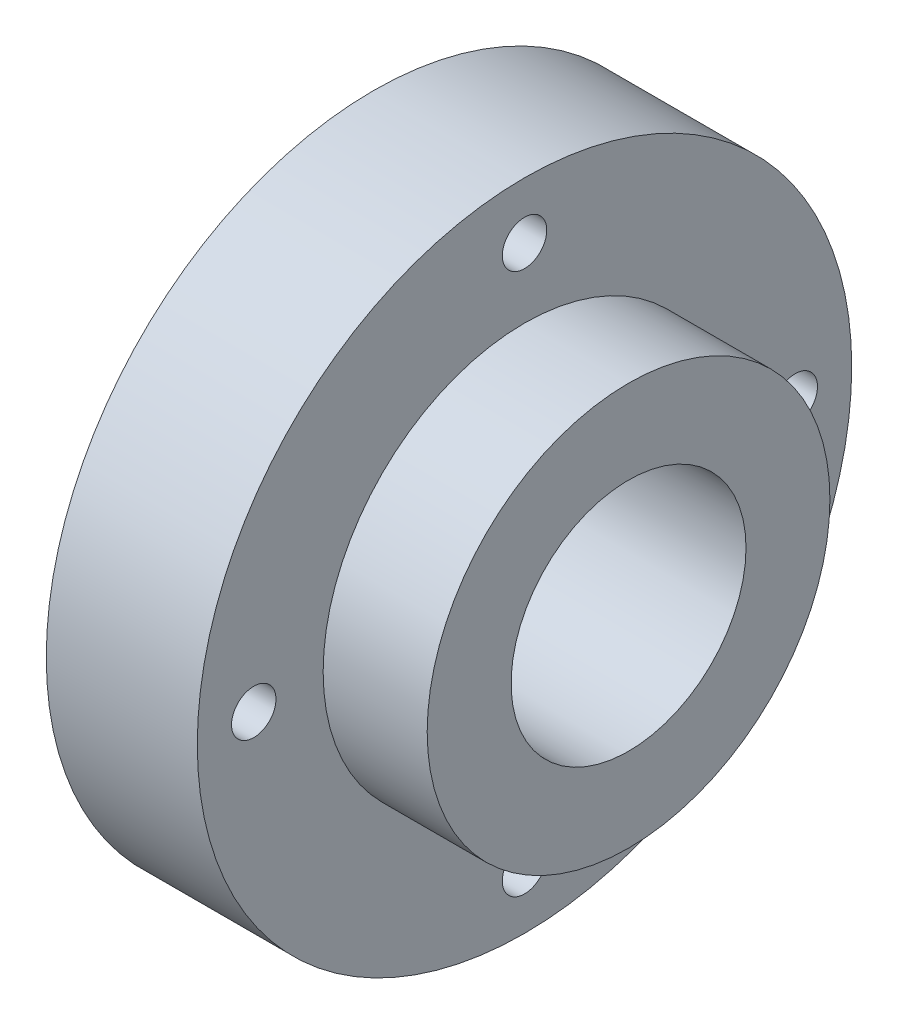
ISO-10303-21;
HEADER;
FILE_DESCRIPTION(('STEP AP214'),'2;1');
FILE_NAME('part.step','',(''),(''),'','','');
FILE_SCHEMA(('AUTOMOTIVE_DESIGN { 1 0 10303 214 1 1 1 1 }'));
ENDSEC;
DATA;
#1=APPLICATION_CONTEXT('core data for automotive mechanical design processes');
#2=APPLICATION_PROTOCOL_DEFINITION('international standard','automotive_design',2000,#1);
#3=PRODUCT_CONTEXT('',#1,'mechanical');
#4=PRODUCT('Part','Part','',(#3));
#5=PRODUCT_RELATED_PRODUCT_CATEGORY('part','',(#4));
#6=PRODUCT_DEFINITION_FORMATION('','',#4);
#7=PRODUCT_DEFINITION_CONTEXT('part definition',#1,'design');
#8=PRODUCT_DEFINITION('design','',#6,#7);
#9=PRODUCT_DEFINITION_SHAPE('','',#8);
#10=(LENGTH_UNIT() NAMED_UNIT(*) SI_UNIT(.MILLI.,.METRE.));
#11=(NAMED_UNIT(*) PLANE_ANGLE_UNIT() SI_UNIT($,.RADIAN.));
#12=(NAMED_UNIT(*) SI_UNIT($,.STERADIAN.) SOLID_ANGLE_UNIT());
#13=UNCERTAINTY_MEASURE_WITH_UNIT(LENGTH_MEASURE(1.E-05),#10,'distance_accuracy_value','');
#14=(GEOMETRIC_REPRESENTATION_CONTEXT(3) GLOBAL_UNCERTAINTY_ASSIGNED_CONTEXT((#13)) GLOBAL_UNIT_ASSIGNED_CONTEXT((#10,
#11,#12)) REPRESENTATION_CONTEXT('',''));
#15=CARTESIAN_POINT('',(0.,0.,0.));
#16=DIRECTION('',(0.,0.,1.));
#17=DIRECTION('',(1.,0.,0.));
#18=AXIS2_PLACEMENT_3D('',#15,#16,#17);
#19=CARTESIAN_POINT('',(-295.6,0.,0.));
#20=DIRECTION('',(1.,0.,0.));
#21=DIRECTION('',(0.,0.,-1.));
#22=AXIS2_PLACEMENT_3D('',#19,#20,#21);
#23=CYLINDRICAL_SURFACE('',#22,14.);
#24=CARTESIAN_POINT('',(21.4,0.,0.));
#25=DIRECTION('',(1.,0.,0.));
#26=DIRECTION('',(0.,0.,-1.));
#27=AXIS2_PLACEMENT_3D('',#24,#25,#26);
#28=CIRCLE('',#27,14.);
#29=CARTESIAN_POINT('',(21.4,0.,-14.));
#30=VERTEX_POINT('',#29);
#31=EDGE_CURVE('E67',#30,#30,#28,.T.);
#32=ORIENTED_EDGE('',*,*,#31,.T.);
#33=EDGE_LOOP('',(#32));
#34=FACE_BOUND('',#33,.T.);
#35=CARTESIAN_POINT('',(-3.,0.,0.));
#36=DIRECTION('',(-1.,0.,0.));
#37=DIRECTION('',(0.,0.,1.));
#38=AXIS2_PLACEMENT_3D('',#35,#36,#37);
#39=CIRCLE('',#38,14.);
#40=CARTESIAN_POINT('',(-3.,0.,14.));
#41=VERTEX_POINT('',#40);
#42=EDGE_CURVE('E44',#41,#41,#39,.F.);
#43=ORIENTED_EDGE('',*,*,#42,.F.);
#44=EDGE_LOOP('',(#43));
#45=FACE_BOUND('',#44,.T.);
#46=ADVANCED_FACE('F41',(#34,#45),#23,.F.);
#47=CARTESIAN_POINT('',(-295.6,0.,32.2694333599353));
#48=DIRECTION('',(1.,0.,0.));
#49=DIRECTION('',(0.,0.,-1.));
#50=AXIS2_PLACEMENT_3D('',#47,#48,#49);
#51=CYLINDRICAL_SURFACE('',#50,2.65000000000059);
#52=CARTESIAN_POINT('',(9.00000000000001,0.,32.2694333599353));
#53=DIRECTION('',(-1.,0.,0.));
#54=DIRECTION('',(0.,0.,1.));
#55=AXIS2_PLACEMENT_3D('',#52,#53,#54);
#56=CIRCLE('',#55,2.65000000000059);
#57=CARTESIAN_POINT('',(9.00000000000001,0.,34.9194333599359));
#58=VERTEX_POINT('',#57);
#59=EDGE_CURVE('E73',#58,#58,#56,.T.);
#60=ORIENTED_EDGE('',*,*,#59,.F.);
#61=EDGE_LOOP('',(#60));
#62=FACE_BOUND('',#61,.T.);
#63=CARTESIAN_POINT('',(-5.,0.,32.2694333599353));
#64=DIRECTION('',(-1.,0.,0.));
#65=DIRECTION('',(0.,0.,1.));
#66=AXIS2_PLACEMENT_3D('',#63,#64,#65);
#67=CIRCLE('',#66,2.65000000000059);
#68=CARTESIAN_POINT('',(-5.,0.,34.9194333599359));
#69=VERTEX_POINT('',#68);
#70=EDGE_CURVE('E70',#69,#69,#67,.F.);
#71=ORIENTED_EDGE('',*,*,#70,.F.);
#72=EDGE_LOOP('',(#71));
#73=FACE_BOUND('',#72,.T.);
#74=ADVANCED_FACE('F120',(#62,#73),#51,.F.);
#75=CARTESIAN_POINT('',(-295.6,-32.2694333599353,0.));
#76=DIRECTION('',(1.,0.,0.));
#77=DIRECTION('',(0.,0.,-1.));
#78=AXIS2_PLACEMENT_3D('',#75,#76,#77);
#79=CYLINDRICAL_SURFACE('',#78,2.65000000000048);
#80=CARTESIAN_POINT('',(9.00000000000001,-32.2694333599353,0.));
#81=DIRECTION('',(-1.,0.,0.));
#82=DIRECTION('',(0.,0.,1.));
#83=AXIS2_PLACEMENT_3D('',#80,#81,#82);
#84=CIRCLE('',#83,2.65000000000048);
#85=CARTESIAN_POINT('',(9.00000000000001,-32.2694333599353,2.65000000000048));
#86=VERTEX_POINT('',#85);
#87=EDGE_CURVE('E76',#86,#86,#84,.T.);
#88=ORIENTED_EDGE('',*,*,#87,.F.);
#89=EDGE_LOOP('',(#88));
#90=FACE_BOUND('',#89,.T.);
#91=CARTESIAN_POINT('',(-5.,-32.2694333599353,0.));
#92=DIRECTION('',(-1.,0.,0.));
#93=DIRECTION('',(0.,0.,1.));
#94=AXIS2_PLACEMENT_3D('',#91,#92,#93);
#95=CIRCLE('',#94,2.65000000000048);
#96=CARTESIAN_POINT('',(-5.,-32.2694333599353,2.65000000000048));
#97=VERTEX_POINT('',#96);
#98=EDGE_CURVE('E63',#97,#97,#95,.F.);
#99=ORIENTED_EDGE('',*,*,#98,.F.);
#100=EDGE_LOOP('',(#99));
#101=FACE_BOUND('',#100,.T.);
#102=ADVANCED_FACE('F125',(#90,#101),#79,.F.);
#103=CARTESIAN_POINT('',(-295.6,0.,-32.2694333599353));
#104=DIRECTION('',(1.,0.,0.));
#105=DIRECTION('',(0.,0.,-1.));
#106=AXIS2_PLACEMENT_3D('',#103,#104,#105);
#107=CYLINDRICAL_SURFACE('',#106,2.65000000000037);
#108=CARTESIAN_POINT('',(9.00000000000001,0.,-32.2694333599353));
#109=DIRECTION('',(-1.,0.,0.));
#110=DIRECTION('',(0.,0.,1.));
#111=AXIS2_PLACEMENT_3D('',#108,#109,#110);
#112=CIRCLE('',#111,2.65000000000037);
#113=CARTESIAN_POINT('',(9.00000000000001,0.,-29.619433359935));
#114=VERTEX_POINT('',#113);
#115=EDGE_CURVE('E86',#114,#114,#112,.T.);
#116=ORIENTED_EDGE('',*,*,#115,.F.);
#117=EDGE_LOOP('',(#116));
#118=FACE_BOUND('',#117,.T.);
#119=CARTESIAN_POINT('',(-5.,0.,-32.2694333599353));
#120=DIRECTION('',(-1.,0.,0.));
#121=DIRECTION('',(0.,0.,1.));
#122=AXIS2_PLACEMENT_3D('',#119,#120,#121);
#123=CIRCLE('',#122,2.65000000000037);
#124=CARTESIAN_POINT('',(-5.,0.,-29.619433359935));
#125=VERTEX_POINT('',#124);
#126=EDGE_CURVE('E62',#125,#125,#123,.F.);
#127=ORIENTED_EDGE('',*,*,#126,.F.);
#128=EDGE_LOOP('',(#127));
#129=FACE_BOUND('',#128,.T.);
#130=ADVANCED_FACE('F130',(#118,#129),#107,.F.);
#131=CARTESIAN_POINT('',(-295.6,32.2694333599353,0.));
#132=DIRECTION('',(1.,0.,0.));
#133=DIRECTION('',(0.,0.,-1.));
#134=AXIS2_PLACEMENT_3D('',#131,#132,#133);
#135=CYLINDRICAL_SURFACE('',#134,2.65000000000026);
#136=CARTESIAN_POINT('',(9.00000000000001,32.2694333599353,0.));
#137=DIRECTION('',(-1.,0.,0.));
#138=DIRECTION('',(0.,0.,1.));
#139=AXIS2_PLACEMENT_3D('',#136,#137,#138);
#140=CIRCLE('',#139,2.65000000000026);
#141=CARTESIAN_POINT('',(9.00000000000001,32.2694333599353,2.65000000000025));
#142=VERTEX_POINT('',#141);
#143=EDGE_CURVE('E87',#142,#142,#140,.T.);
#144=ORIENTED_EDGE('',*,*,#143,.F.);
#145=EDGE_LOOP('',(#144));
#146=FACE_BOUND('',#145,.T.);
#147=CARTESIAN_POINT('',(-5.,32.2694333599353,0.));
#148=DIRECTION('',(-1.,0.,0.));
#149=DIRECTION('',(0.,0.,1.));
#150=AXIS2_PLACEMENT_3D('',#147,#148,#149);
#151=CIRCLE('',#150,2.65000000000026);
#152=CARTESIAN_POINT('',(-5.,32.2694333599353,2.65000000000025));
#153=VERTEX_POINT('',#152);
#154=EDGE_CURVE('E59',#153,#153,#151,.F.);
#155=ORIENTED_EDGE('',*,*,#154,.F.);
#156=EDGE_LOOP('',(#155));
#157=FACE_BOUND('',#156,.T.);
#158=ADVANCED_FACE('F128',(#146,#157),#135,.F.);
#159=CARTESIAN_POINT('',(6.59999999999999,0.,0.));
#160=DIRECTION('',(-1.,0.,0.));
#161=DIRECTION('',(0.,0.,1.));
#162=AXIS2_PLACEMENT_3D('',#159,#160,#161);
#163=CYLINDRICAL_SURFACE('',#162,39.);
#164=CARTESIAN_POINT('',(9.,0.,0.));
#165=DIRECTION('',(-1.,0.,0.));
#166=DIRECTION('',(0.,0.,1.));
#167=AXIS2_PLACEMENT_3D('',#164,#165,#166);
#168=CIRCLE('',#167,39.);
#169=CARTESIAN_POINT('',(9.,0.,39.));
#170=VERTEX_POINT('',#169);
#171=EDGE_CURVE('E10',#170,#170,#168,.T.);
#172=ORIENTED_EDGE('',*,*,#171,.T.);
#173=EDGE_LOOP('',(#172));
#174=FACE_BOUND('',#173,.T.);
#175=CARTESIAN_POINT('',(-9.,0.,0.));
#176=DIRECTION('',(-1.,0.,0.));
#177=DIRECTION('',(0.,0.,1.));
#178=AXIS2_PLACEMENT_3D('',#175,#176,#177);
#179=CIRCLE('',#178,39.);
#180=CARTESIAN_POINT('',(-9.,0.,39.));
#181=VERTEX_POINT('',#180);
#182=EDGE_CURVE('E95',#181,#181,#179,.T.);
#183=ORIENTED_EDGE('',*,*,#182,.F.);
#184=EDGE_LOOP('',(#183));
#185=FACE_BOUND('',#184,.T.);
#186=ADVANCED_FACE('F43',(#174,#185),#163,.T.);
#187=CARTESIAN_POINT('',(9.,0.,0.));
#188=DIRECTION('',(-1.,0.,0.));
#189=DIRECTION('',(0.,0.,1.));
#190=AXIS2_PLACEMENT_3D('',#187,#188,#189);
#191=PLANE('',#190);
#192=ORIENTED_EDGE('',*,*,#143,.T.);
#193=EDGE_LOOP('',(#192));
#194=FACE_BOUND('',#193,.T.);
#195=ORIENTED_EDGE('',*,*,#115,.T.);
#196=EDGE_LOOP('',(#195));
#197=FACE_BOUND('',#196,.T.);
#198=ORIENTED_EDGE('',*,*,#87,.T.);
#199=EDGE_LOOP('',(#198));
#200=FACE_BOUND('',#199,.T.);
#201=ORIENTED_EDGE('',*,*,#59,.T.);
#202=EDGE_LOOP('',(#201));
#203=FACE_BOUND('',#202,.T.);
#204=ORIENTED_EDGE('',*,*,#171,.F.);
#205=EDGE_LOOP('',(#204));
#206=FACE_BOUND('',#205,.T.);
#207=CARTESIAN_POINT('',(9.,0.,0.));
#208=DIRECTION('',(-1.,0.,0.));
#209=DIRECTION('',(0.,0.,1.));
#210=AXIS2_PLACEMENT_3D('',#207,#208,#209);
#211=CIRCLE('',#210,24.);
#212=CARTESIAN_POINT('',(9.,0.,24.));
#213=VERTEX_POINT('',#212);
#214=EDGE_CURVE('E47',#213,#213,#211,.T.);
#215=ORIENTED_EDGE('',*,*,#214,.T.);
#216=EDGE_LOOP('',(#215));
#217=FACE_BOUND('',#216,.T.);
#218=ADVANCED_FACE('F112',(#194,#197,#200,#203,#206,#217),#191,.F.);
#219=CARTESIAN_POINT('',(6.59999999999999,0.,0.));
#220=DIRECTION('',(-1.,0.,0.));
#221=DIRECTION('',(0.,0.,1.));
#222=AXIS2_PLACEMENT_3D('',#219,#220,#221);
#223=CYLINDRICAL_SURFACE('',#222,24.);
#224=CARTESIAN_POINT('',(21.4,0.,0.));
#225=DIRECTION('',(-1.,0.,0.));
#226=DIRECTION('',(0.,0.,1.));
#227=AXIS2_PLACEMENT_3D('',#224,#225,#226);
#228=CIRCLE('',#227,24.);
#229=CARTESIAN_POINT('',(21.4,0.,24.));
#230=VERTEX_POINT('',#229);
#231=EDGE_CURVE('E53',#230,#230,#228,.T.);
#232=ORIENTED_EDGE('',*,*,#231,.T.);
#233=EDGE_LOOP('',(#232));
#234=FACE_BOUND('',#233,.T.);
#235=ORIENTED_EDGE('',*,*,#214,.F.);
#236=EDGE_LOOP('',(#235));
#237=FACE_BOUND('',#236,.T.);
#238=ADVANCED_FACE('F97',(#234,#237),#223,.T.);
#239=CARTESIAN_POINT('',(21.4,0.,0.));
#240=DIRECTION('',(-1.,0.,0.));
#241=DIRECTION('',(0.,0.,1.));
#242=AXIS2_PLACEMENT_3D('',#239,#240,#241);
#243=PLANE('',#242);
#244=ORIENTED_EDGE('',*,*,#31,.F.);
#245=EDGE_LOOP('',(#244));
#246=FACE_BOUND('',#245,.T.);
#247=ORIENTED_EDGE('',*,*,#231,.F.);
#248=EDGE_LOOP('',(#247));
#249=FACE_BOUND('',#248,.T.);
#250=ADVANCED_FACE('F99',(#246,#249),#243,.F.);
#251=CARTESIAN_POINT('',(-9.,0.,0.));
#252=DIRECTION('',(-1.,0.,0.));
#253=DIRECTION('',(0.,0.,1.));
#254=AXIS2_PLACEMENT_3D('',#251,#252,#253);
#255=PLANE('',#254);
#256=CARTESIAN_POINT('',(-9.,0.,0.));
#257=DIRECTION('',(-1.,0.,0.));
#258=DIRECTION('',(0.,0.,1.));
#259=AXIS2_PLACEMENT_3D('',#256,#257,#258);
#260=CIRCLE('',#259,19.);
#261=CARTESIAN_POINT('',(-9.,0.,19.));
#262=VERTEX_POINT('',#261);
#263=EDGE_CURVE('E184',#262,#262,#260,.T.);
#264=ORIENTED_EDGE('',*,*,#263,.F.);
#265=EDGE_LOOP('',(#264));
#266=FACE_BOUND('',#265,.T.);
#267=CARTESIAN_POINT('',(-9.,32.2694333599353,0.));
#268=DIRECTION('',(-1.,0.,0.));
#269=DIRECTION('',(0.,0.,1.));
#270=AXIS2_PLACEMENT_3D('',#267,#268,#269);
#271=CIRCLE('',#270,3.50000000000027);
#272=CARTESIAN_POINT('',(-9.,32.2694333599353,3.50000000000027));
#273=VERTEX_POINT('',#272);
#274=EDGE_CURVE('E195',#273,#273,#271,.T.);
#275=ORIENTED_EDGE('',*,*,#274,.F.);
#276=EDGE_LOOP('',(#275));
#277=FACE_BOUND('',#276,.T.);
#278=CARTESIAN_POINT('',(-9.,0.,-32.2694333599353));
#279=DIRECTION('',(-1.,0.,0.));
#280=DIRECTION('',(0.,0.,1.));
#281=AXIS2_PLACEMENT_3D('',#278,#279,#280);
#282=CIRCLE('',#281,3.49999999999853);
#283=CARTESIAN_POINT('',(-9.,0.,-28.7694333599368));
#284=VERTEX_POINT('',#283);
#285=EDGE_CURVE('E198',#284,#284,#282,.T.);
#286=ORIENTED_EDGE('',*,*,#285,.F.);
#287=EDGE_LOOP('',(#286));
#288=FACE_BOUND('',#287,.T.);
#289=CARTESIAN_POINT('',(-9.,-32.2694333599353,0.));
#290=DIRECTION('',(-1.,0.,0.));
#291=DIRECTION('',(0.,0.,1.));
#292=AXIS2_PLACEMENT_3D('',#289,#290,#291);
#293=CIRCLE('',#292,3.49999999999799);
#294=CARTESIAN_POINT('',(-9.,-32.2694333599353,3.49999999999799));
#295=VERTEX_POINT('',#294);
#296=EDGE_CURVE('E204',#295,#295,#293,.T.);
#297=ORIENTED_EDGE('',*,*,#296,.F.);
#298=EDGE_LOOP('',(#297));
#299=FACE_BOUND('',#298,.T.);
#300=CARTESIAN_POINT('',(-9.,0.,32.2694333599353));
#301=DIRECTION('',(-1.,0.,0.));
#302=DIRECTION('',(0.,0.,1.));
#303=AXIS2_PLACEMENT_3D('',#300,#301,#302);
#304=CIRCLE('',#303,3.49999999999973);
#305=CARTESIAN_POINT('',(-9.,0.,35.7694333599351));
#306=VERTEX_POINT('',#305);
#307=EDGE_CURVE('E82',#306,#306,#304,.T.);
#308=ORIENTED_EDGE('',*,*,#307,.F.);
#309=EDGE_LOOP('',(#308));
#310=FACE_BOUND('',#309,.T.);
#311=ORIENTED_EDGE('',*,*,#182,.T.);
#312=EDGE_LOOP('',(#311));
#313=FACE_BOUND('',#312,.T.);
#314=ADVANCED_FACE('F105',(#266,#277,#288,#299,#310,#313),#255,.T.);
#315=CARTESIAN_POINT('',(-5.,32.2694333599353,0.));
#316=DIRECTION('',(-1.,0.,0.));
#317=DIRECTION('',(0.,0.,1.));
#318=AXIS2_PLACEMENT_3D('',#315,#316,#317);
#319=PLANE('',#318);
#320=CARTESIAN_POINT('',(-5.,32.2694333599353,0.));
#321=DIRECTION('',(-1.,0.,0.));
#322=DIRECTION('',(0.,0.,1.));
#323=AXIS2_PLACEMENT_3D('',#320,#321,#322);
#324=CIRCLE('',#323,3.50000000000027);
#325=CARTESIAN_POINT('',(-5.,32.2694333599353,3.50000000000027));
#326=VERTEX_POINT('',#325);
#327=EDGE_CURVE('E65',#326,#326,#324,.T.);
#328=ORIENTED_EDGE('',*,*,#327,.T.);
#329=EDGE_LOOP('',(#328));
#330=FACE_BOUND('',#329,.T.);
#331=ORIENTED_EDGE('',*,*,#154,.T.);
#332=EDGE_LOOP('',(#331));
#333=FACE_BOUND('',#332,.T.);
#334=ADVANCED_FACE('F109',(#330,#333),#319,.T.);
#335=CARTESIAN_POINT('',(-5.,32.2694333599353,0.));
#336=DIRECTION('',(-1.,0.,0.));
#337=DIRECTION('',(0.,0.,1.));
#338=AXIS2_PLACEMENT_3D('',#335,#336,#337);
#339=CYLINDRICAL_SURFACE('',#338,3.50000000000027);
#340=ORIENTED_EDGE('',*,*,#327,.F.);
#341=EDGE_LOOP('',(#340));
#342=FACE_BOUND('',#341,.T.);
#343=ORIENTED_EDGE('',*,*,#274,.T.);
#344=EDGE_LOOP('',(#343));
#345=FACE_BOUND('',#344,.T.);
#346=ADVANCED_FACE('F163',(#342,#345),#339,.F.);
#347=CARTESIAN_POINT('',(-5.,0.,-32.2694333599353));
#348=DIRECTION('',(-1.,0.,0.));
#349=DIRECTION('',(0.,0.,1.));
#350=AXIS2_PLACEMENT_3D('',#347,#348,#349);
#351=PLANE('',#350);
#352=CARTESIAN_POINT('',(-5.,0.,-32.2694333599353));
#353=DIRECTION('',(-1.,0.,0.));
#354=DIRECTION('',(0.,0.,1.));
#355=AXIS2_PLACEMENT_3D('',#352,#353,#354);
#356=CIRCLE('',#355,3.49999999999853);
#357=CARTESIAN_POINT('',(-5.,0.,-28.7694333599368));
#358=VERTEX_POINT('',#357);
#359=EDGE_CURVE('E193',#358,#358,#356,.T.);
#360=ORIENTED_EDGE('',*,*,#359,.T.);
#361=EDGE_LOOP('',(#360));
#362=FACE_BOUND('',#361,.T.);
#363=ORIENTED_EDGE('',*,*,#126,.T.);
#364=EDGE_LOOP('',(#363));
#365=FACE_BOUND('',#364,.T.);
#366=ADVANCED_FACE('F160',(#362,#365),#351,.T.);
#367=CARTESIAN_POINT('',(-5.,0.,-32.2694333599353));
#368=DIRECTION('',(-1.,0.,0.));
#369=DIRECTION('',(0.,0.,1.));
#370=AXIS2_PLACEMENT_3D('',#367,#368,#369);
#371=CYLINDRICAL_SURFACE('',#370,3.49999999999853);
#372=ORIENTED_EDGE('',*,*,#359,.F.);
#373=EDGE_LOOP('',(#372));
#374=FACE_BOUND('',#373,.T.);
#375=ORIENTED_EDGE('',*,*,#285,.T.);
#376=EDGE_LOOP('',(#375));
#377=FACE_BOUND('',#376,.T.);
#378=ADVANCED_FACE('F153',(#374,#377),#371,.F.);
#379=CARTESIAN_POINT('',(-5.,-32.2694333599353,0.));
#380=DIRECTION('',(-1.,0.,0.));
#381=DIRECTION('',(0.,0.,1.));
#382=AXIS2_PLACEMENT_3D('',#379,#380,#381);
#383=PLANE('',#382);
#384=CARTESIAN_POINT('',(-5.,-32.2694333599353,0.));
#385=DIRECTION('',(-1.,0.,0.));
#386=DIRECTION('',(0.,0.,1.));
#387=AXIS2_PLACEMENT_3D('',#384,#385,#386);
#388=CIRCLE('',#387,3.49999999999799);
#389=CARTESIAN_POINT('',(-5.,-32.2694333599353,3.49999999999799));
#390=VERTEX_POINT('',#389);
#391=EDGE_CURVE('E202',#390,#390,#388,.T.);
#392=ORIENTED_EDGE('',*,*,#391,.T.);
#393=EDGE_LOOP('',(#392));
#394=FACE_BOUND('',#393,.T.);
#395=ORIENTED_EDGE('',*,*,#98,.T.);
#396=EDGE_LOOP('',(#395));
#397=FACE_BOUND('',#396,.T.);
#398=ADVANCED_FACE('F146',(#394,#397),#383,.T.);
#399=CARTESIAN_POINT('',(-5.,-32.2694333599353,0.));
#400=DIRECTION('',(-1.,0.,0.));
#401=DIRECTION('',(0.,0.,1.));
#402=AXIS2_PLACEMENT_3D('',#399,#400,#401);
#403=CYLINDRICAL_SURFACE('',#402,3.49999999999799);
#404=ORIENTED_EDGE('',*,*,#391,.F.);
#405=EDGE_LOOP('',(#404));
#406=FACE_BOUND('',#405,.T.);
#407=ORIENTED_EDGE('',*,*,#296,.T.);
#408=EDGE_LOOP('',(#407));
#409=FACE_BOUND('',#408,.T.);
#410=ADVANCED_FACE('F143',(#406,#409),#403,.F.);
#411=CARTESIAN_POINT('',(-5.,0.,32.2694333599353));
#412=DIRECTION('',(-1.,0.,0.));
#413=DIRECTION('',(0.,0.,1.));
#414=AXIS2_PLACEMENT_3D('',#411,#412,#413);
#415=PLANE('',#414);
#416=CARTESIAN_POINT('',(-5.,0.,32.2694333599353));
#417=DIRECTION('',(-1.,0.,0.));
#418=DIRECTION('',(0.,0.,1.));
#419=AXIS2_PLACEMENT_3D('',#416,#417,#418);
#420=CIRCLE('',#419,3.49999999999973);
#421=CARTESIAN_POINT('',(-5.,0.,35.7694333599351));
#422=VERTEX_POINT('',#421);
#423=EDGE_CURVE('E183',#422,#422,#420,.T.);
#424=ORIENTED_EDGE('',*,*,#423,.T.);
#425=EDGE_LOOP('',(#424));
#426=FACE_BOUND('',#425,.T.);
#427=ORIENTED_EDGE('',*,*,#70,.T.);
#428=EDGE_LOOP('',(#427));
#429=FACE_BOUND('',#428,.T.);
#430=ADVANCED_FACE('F142',(#426,#429),#415,.T.);
#431=CARTESIAN_POINT('',(-5.,0.,32.2694333599353));
#432=DIRECTION('',(-1.,0.,0.));
#433=DIRECTION('',(0.,0.,1.));
#434=AXIS2_PLACEMENT_3D('',#431,#432,#433);
#435=CYLINDRICAL_SURFACE('',#434,3.49999999999973);
#436=ORIENTED_EDGE('',*,*,#423,.F.);
#437=EDGE_LOOP('',(#436));
#438=FACE_BOUND('',#437,.T.);
#439=ORIENTED_EDGE('',*,*,#307,.T.);
#440=EDGE_LOOP('',(#439));
#441=FACE_BOUND('',#440,.T.);
#442=ADVANCED_FACE('F138',(#438,#441),#435,.F.);
#443=CARTESIAN_POINT('',(-3.,0.,0.));
#444=DIRECTION('',(-1.,0.,0.));
#445=DIRECTION('',(0.,0.,1.));
#446=AXIS2_PLACEMENT_3D('',#443,#444,#445);
#447=PLANE('',#446);
#448=CARTESIAN_POINT('',(-3.,0.,0.));
#449=DIRECTION('',(-1.,0.,0.));
#450=DIRECTION('',(0.,0.,1.));
#451=AXIS2_PLACEMENT_3D('',#448,#449,#450);
#452=CIRCLE('',#451,19.);
#453=CARTESIAN_POINT('',(-3.,0.,19.));
#454=VERTEX_POINT('',#453);
#455=EDGE_CURVE('E179',#454,#454,#452,.T.);
#456=ORIENTED_EDGE('',*,*,#455,.T.);
#457=EDGE_LOOP('',(#456));
#458=FACE_BOUND('',#457,.T.);
#459=ORIENTED_EDGE('',*,*,#42,.T.);
#460=EDGE_LOOP('',(#459));
#461=FACE_BOUND('',#460,.T.);
#462=ADVANCED_FACE('F136',(#458,#461),#447,.T.);
#463=CARTESIAN_POINT('',(-3.,0.,0.));
#464=DIRECTION('',(-1.,0.,0.));
#465=DIRECTION('',(0.,0.,1.));
#466=AXIS2_PLACEMENT_3D('',#463,#464,#465);
#467=CYLINDRICAL_SURFACE('',#466,19.);
#468=ORIENTED_EDGE('',*,*,#455,.F.);
#469=EDGE_LOOP('',(#468));
#470=FACE_BOUND('',#469,.T.);
#471=ORIENTED_EDGE('',*,*,#263,.T.);
#472=EDGE_LOOP('',(#471));
#473=FACE_BOUND('',#472,.T.);
#474=ADVANCED_FACE('F169',(#470,#473),#467,.F.);
#475=CLOSED_SHELL('',(#46,#74,#102,#130,#158,#186,#218,#238,#250,#314,#334,#346,#366,#378,#398,
#410,#430,#442,#462,#474));
#476=MANIFOLD_SOLID_BREP('B2',#475);
#477=ADVANCED_BREP_SHAPE_REPRESENTATION('',(#18,#476),#14);
#478=SHAPE_DEFINITION_REPRESENTATION(#9,#477);
ENDSEC;
END-ISO-10303-21;
